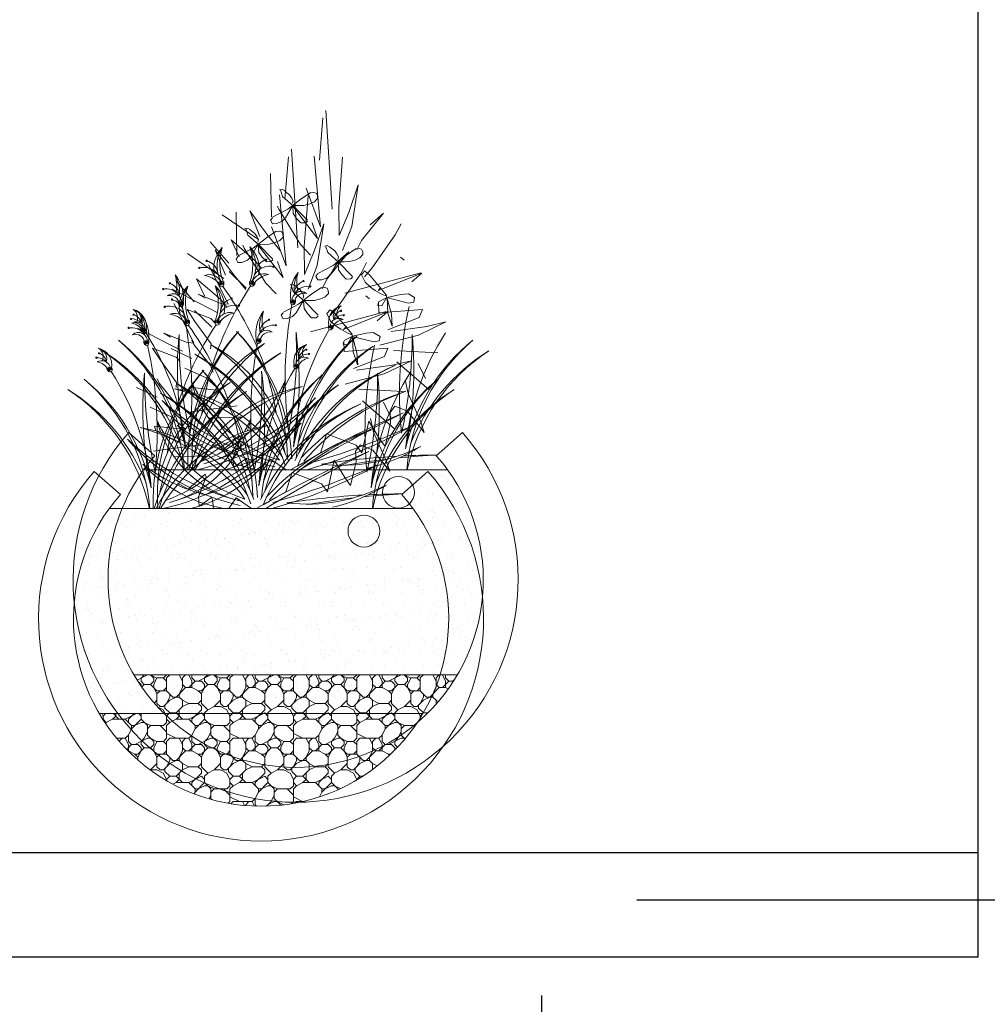
# Model space of a CAD drawing. Units: inches. Extents: x 89 to 490, y -59 to 378.
# Tile 15 of 20: x 429 to 460, y -28 to 3. Entities that reach past the tile are written whole.
import ezdxf

# ---------------------------------------------------------------- set-up
doc = ezdxf.new("R2010")
doc.units = ezdxf.units.IN
doc.header["$MEASUREMENT"] = 0
for name, color, linetype, lineweight in [('A-ANNO-DIMS', 2, 'Continuous', 18), ('L-PLNT', 94, 'Continuous', 18), ('L-PLNT-EDGE', 31, 'Continuous', 25)]:
    doc.layers.add(name, color=color, linetype=linetype, lineweight=lineweight)
doc.layers.add('fl', color=73, linetype='Continuous', lineweight=9, true_color=0xa3d166)
doc.styles.get("Standard").update_dxf_attribs({"font": 'arial.ttf'})
doc.dimstyles.get("Standard").update_dxf_attribs({"dimtxt": 6, "dimasz": 4, "dimexe": 3, "dimexo": 3, "dimgap": 0.09, "dimtad": 0, "dimtih": 1, "dimtoh": 1, "dimdec": 1, "dimzin": 0, "dimdsep": 46, "dimlunit": 3, "dimtxsty": 'Standard', "dimcen": 0.09, "dimadec": 0, "dimazin": 0, "dimtfac": 1, "dimtdec": 1, "dimtofl": 0, "dimtmove": 0, "dimatfit": 3, "dimfxl": 1, "dimtolj": 1, "dimtzin": 0, "dimarcsym": 0})

# ---------------------------------------------------------------- blocks, each defined once
blk = doc.blocks.new('1')
at = {"layer": 'fl'}
h = blk.add_hatch(dxfattribs=at)
h.set_pattern_fill('AR-SAND', color=256, scale=570.105873, style=0)
h.set_pattern_definition([(37.5, (-3711399.5, -832187.1), (-35.91288, 1098.49355), [0, -866.56093, 0, -969.17998, 0, -926.42204]), (7.5, (-3711399.5, -832187.1), (1008.9601, 1608.92205), [0, -467.48682, 0, -781.04505, 0, -299.30558]), (327.5, (-3712100.7, -832187.1), (1775.39056, 3.22626), [0, -285.05294, 0, -1026.19057, 0, -1339.7488]), (317.5, (-3712100.7, -832187.1), (1713.81043, 500.368), [0, -142.52647, 0, -672.72493, 0, -769.64293])])
h.paths.add_polyline_path([(227046, 19995, 0.298047), (226601, 10772), (241144, 10772, 0.298047), (240699, 19995)])
h.paths.add_polyline_path([(237778, 18976, -1), (239209, 18976, -1)], flags=16)
h = blk.add_hatch(dxfattribs=at)
h.set_pattern_fill('GHIAIA2', color=256, scale=2850.529365, style=0, pattern_type=2)
h.set_pattern_definition([(0, (-3711257, -832187), (2850.5294, 2850.5294), [855.1588, -997.6853, 142.5265, -855.1588]), (0, (-3710116.7, -831617), (2850.5294, 2850.5294), [142.5265, -712.6323, 570.1059, -1425.2647]), (0, (-3709689.2, -831474.5), (2850.5294, 2850.5294), [142.5265, -2708.0029]), (0, (-3710972, -831332), (2850.5294, 2850.5294), [570.1059, -2280.4235]), (0, (-3711257, -831047), (2850.5294, 2850.5294), [285.053, -2565.4764]), (0, (-3709261.6, -830761.8), (2850.5294, 2850.5294), [285.0529, -142.5265, 142.5265, -2280.4235]), (0, (-3710401.8, -830619.3), (2850.5294, 2850.5294), [427.5794, -2422.95]), (0, (-3711114.4, -830334.2), (2850.5294, 2850.5294), [285.053, -2565.4764]), (0, (-3709974.2, -830049.2), (2850.5294, 2850.5294), [142.5265, -855.1588, 427.5794, -1425.2647]), (0, (-3710544.3, -829906.7), (2850.5294, 2850.5294), [285.053, -2565.4764]), (0, (-3709546.6, -829764), (2850.5294, 2850.5294), [285.053, -2565.4764]), (0, (-3710116.7, -829621.6), (2850.5294, 2850.5294), [285.053, -2565.4764]), (0, (-3708976.5, -829479), (2850.5294, 2850.5294), [285.053, -2565.4764]), (90, (-3711399.5, -832187), (-2850.5294, 2850.5294), [570.1059, -142.5265, 285.05294, -1140.21175, 570.1059, -142.5265]), (90, (-3711257, -830334.2), (-2850.5294, 2850.5294), [142.5265, -2708.0029]), (90, (-3710829.4, -831189.4), (-2850.5294, 2850.5294), [285.0529, -570.1059, 142.5265, -1852.8441]), (90, (-3710686.9, -830761.8), (-2850.5294, 2850.5294), [285.0529, -570.1059, 427.5794, -1567.7912]), (90, (-3710259.3, -831474.5), (-2850.5294, 2850.5294), [142.5265, -1425.2647, 285.05294, -142.5265, 285.05294, -570.1059]), (90, (-3710116.7, -831759.5), (-2850.5294, 2850.5294), [142.5265, -2708.0029]), (90, (-3709831.7, -830904.3), (-2850.5294, 2850.5294), [142.5265, -142.5265, 427.5794, -2137.897]), (90, (-3709689.2, -831332), (-2850.5294, 2850.5294), [285.05294, -1140.21175, 142.5265, -142.5265, 142.5265, -997.6853]), (90, (-3709404, -832044.6), (-2850.5294, 2850.5294), [427.5794, -2422.95]), (90, (-3709119, -829906.7), (-2850.5294, 2850.5294), [142.5265, -142.5265, 142.5265, -2422.95]), (90, (-3708976.5, -830619.3), (-2850.5294, 2850.5294), [427.5794, -2422.95]), (90, (-3708620.2, -830833), (-2850.5294, 2850.5294), [142.5265, -2708.0029]), (45, (-3710401.8, -832187), (3e-13, 2850.5294), [201.561, -3829.6964]), (45, (-3710686.9, -829479), (3e-13, 2850.5294), [201.5609, -604.6828, 604.6828, -2620.3308]), (45, (-3710401.8, -829906.7), (3e-13, 2850.5294), [403.1219, -1007.8143, 201.5609, -2418.7601]), (45, (-3709831.7, -830049.2), (3e-13, 2850.5294), [403.1219, -1410.9408, 201.5609, -2015.6337]), (45, (-3710972, -831332), (3e-13, 2850.5294), [201.561, -3829.6964]), (45, (-3710259.3, -831332), (3e-13, 2850.5294), [604.6885, -3426.5688]), (45, (-3709689.2, -831046.9), (3e-13, 2850.5294), [201.5609, -1209.377, 201.5609, -2418.7584]), (45, (-3709261.6, -830761.8), (3e-13, 2850.5294), [403.1219, -3628.1354]), (45, (-3708691.5, -830761.8), (3e-13, 2850.5294), [403.1219, -3628.1354]), (45, (-3708691.5, -831617), (3e-13, 2850.5294), [201.561, -3829.6964]), (45, (-3708976.5, -830191.7), (3e-13, 2850.5294), [201.561, -3829.6964]), (45, (-3709261.6, -829764.1), (3e-13, 2850.5294), [201.561, -3829.6964]), (45, (-3708691.5, -829479), (3e-13, 2850.5294), [201.561, -3829.6964]), (45, (-3711399.5, -829479), (3e-13, 2850.5294), [201.561, -3829.6964]), (45, (-3709974.2, -830619.3), (3e-13, 2850.5294), [201.561, -3829.6964]), (45, (-3709689.2, -829479), (3e-13, 2850.5294), [201.5609, -1410.9408, 201.5609, -2217.1947]), (45, (-3710972, -831046.9), (3e-13, 2850.5294), [403.1219, -3628.1354]), (45, (-3710972, -830334.2), (3e-13, 2850.5294), [604.6828, -3426.5745]), (135, (-3711257, -831046.9), (-2850.5294, 3e-13), [302.3556, -3728.9016]), (135, (-3709689.2, -831189.4), (-2850.5294, 3e-13), [201.561, -3829.6964]), (135, (-3708834, -830761.8), (-2850.5294, 3e-13), [201.561, -3829.6964]), (135, (-3709831.7, -830191.7), (-2850.5294, 3e-13), [201.561, -3829.6964]), (135, (-3709689.2, -829764.1), (-2850.5294, 3e-13), [201.561, -3829.6964]), (135, (-3710116.7, -829621.6), (-2850.5294, 3e-13), [201.561, -3829.6964]), (135, (-3709546.6, -829764.1), (-2850.5294, 3e-13), [201.561, -3829.6964]), (135, (-3711257, -831474.5), (-2850.5294, 3e-13), [201.561, -3829.6964]), (135, (-3710686.9, -830476.8), (-2850.5294, 3e-13), [201.561, -3829.6964]), (135, (-3710686.9, -831332), (-2850.5294, 3e-13), [403.1219, -3628.1354]), (135, (-3710116.7, -831617), (-2850.5294, 3e-13), [403.1219, -3628.1354]), (135, (-3708976.5, -830049.2), (-2850.5294, 3e-13), [403.1219, -3628.1354]), (135, (-3709831.7, -830761.8), (-2850.5294, 3e-13), [201.561, -3829.6964]), (135, (-3709404.1, -831617), (-2850.5294, 3e-13), [403.1219, -2418.754, 201.5609, -1007.8205]), (135, (-3711114.4, -830334.2), (-2850.5279, 0.0014), [403.1219, -806.2514, 403.1219, -2418.7621]), (135, (-3711399.5, -831902), (-2850.5294, 3e-13), [403.06485, -1007.9472, 403.06485, -1007.9472, 201.5324, -1007.7008]), (26.56505, (-3710401.8, -831331.9), (2850.52937, 1e-07), [637.3784, -318.6892, 318.6892, -5099.2207]), (26.56505, (-3709974.2, -829621.6), (2850.52937, 1e-07), [637.3784, -5736.599]), (26.56505, (-3709974.2, -831617), (2850.52937, 1e-07), [318.6892, -6055.2882]), (26.56505, (-3711257, -831474.5), (2850.52937, 1e-07), [318.6892, -6055.2882]), (26.56505, (-3710686.9, -830761.8), (2850.52937, 1e-07), [318.6892, -6055.2882]), (26.56505, (-3711257, -830476.8), (2850.52937, 1e-07), [318.6892, -6055.2882]), (63.43495, (-3710829.4, -830191.7), (1e-07, 2850.52937), [318.6892, -6055.2882]), (63.43495, (-3709831.7, -830191.7), (1e-07, 2850.52937), [318.6892, -6055.2882]), (63.43495, (-3709546.6, -832187.1), (1e-07, 2850.52937), [318.6892, -6055.2882]), (63.43495, (-3711399.5, -830619.3), (1e-07, 2850.52937), [318.6892, -6055.2882]), (63.43495, (-3710259.3, -832044.6), (1e-07, 2850.52937), [318.6892, -2230.8243, 318.6892, -3505.7748]), (116.56505, (-3710686.9, -829621.6), (-1e-07, 2850.52937), [318.6892, -6055.2882]), (116.56505, (-3708976.5, -830191.7), (-1e-07, 2850.52937), [318.6892, -6055.2882]), (116.56505, (-3710259.3, -829621.6), (-1e-07, 2850.52937), [318.6892, -6055.2882]), (116.56505, (-3711399.5, -831189.4), (-1e-07, 2850.52937), [318.6892, -6055.2882]), (153.43495, (-3709261.6, -831617), (-2850.52937, 1e-07), [318.6892, -6055.2882]), (153.43495, (-3708691.5, -830904.3), (-2850.52937, 1e-07), [318.6892, -6055.2882]), (153.43495, (-3710401.8, -830619.3), (-2850.52937, 1e-07), [318.6892, -6055.2882]), (153.43495, (-3709974.2, -830049.2), (-2850.52937, 1e-07), [318.6892, -6055.2882]), (153.43495, (-3708976.5, -829479.1), (-2850.52937, 1e-07), [318.6892, -6055.2882]), (153.43495, (-3710971.9, -832187.1), (-2850.52937, 1e-07), [478.0338, -5895.9437])])
h.paths.add_polyline_path([(241144, 10772), (226601, 10772, 0.572327)])
for p, q in [((235236, 36144), (235518, 31709)), ((234942, 33904), (235098, 35808)), ((234701, 34090), (234994, 30911)), ((235981, 34049), (235808, 31793)), ((232784, 31366), (232750, 33316)), ((236260, 31559), (236691, 32796)), ((236691, 32796), (236393, 30924)), ((233148, 32578), (233261, 32601)), ((233186, 32582), (233280, 32279)), ((233261, 32601), (233366, 32540)), ((233366, 32540), (233472, 32449)), ((233472, 32449), (233598, 32357)), ((233598, 32357), (233684, 32223)), ((234117, 32169), (234551, 32462)), ((234994, 30911), (234346, 32658)), ((234688, 32459), (234584, 32447)), ((234803, 32430), (234688, 32459)), ((234857, 32317), (234803, 32430)), ((234859, 32192), (234857, 32317)), ((233280, 32279), (233766, 31852)), ((233521, 31704), (234117, 32169)), ((233684, 32223), (233759, 32089)), ((233759, 32089), (233730, 31974)), ((234023, 31865), (234241, 31879)), ((234241, 31879), (234510, 31946)), ((234510, 31946), (234716, 32044)), ((234716, 32044), (234859, 32192)), ((232201, 30339), (230567, 31451)), ((232269, 30478), (231813, 31629)), ((231813, 31629), (232629, 30518)), ((232839, 31348), (233521, 31704)), ((233056, 31838), (233117, 31701)), ((233117, 31701), (234087, 30123)), ((233419, 31324), (233732, 31860)), ((233743, 31839), (234860, 30385)), ((233743, 31839), (233769, 31507)), ((233763, 31871), (234023, 31865)), ((233766, 31852), (234400, 31206)), ((233769, 31507), (233918, 31291)), ((235808, 31793), (235824, 30516)), ((235824, 30516), (236260, 31559)), ((237817, 31528), (236831, 30300)), ((237224, 31008), (237817, 31528)), ((232826, 31324), (232745, 31208)), ((232745, 31208), (232831, 31053)), ((232831, 31053), (233008, 31057)), ((233008, 31057), (233256, 31155)), ((233256, 31155), (233419, 31324)), ((233918, 31291), (234109, 31086)), ((234109, 31086), (234317, 31100)), ((234317, 31100), (234399, 31174)), ((234860, 30385), (234611, 31094)), ((238611, 31055), (238351, 30546)), ((236393, 30924), (235985, 29855)), ((238351, 30546), (237318, 29067)), ((230034, 30240), (230871, 29280)), ((231328, 29557), (230969, 30323)), ((230969, 30323), (232057, 29387)), ((232629, 30518), (233180, 29842)), ((234087, 30123), (234548, 29639)), ((236831, 30300), (236623, 29876)), ((235183, 30051), (235297, 30073)), ((235221, 30054), (235315, 29752)), ((235297, 30073), (235402, 30013)), ((235315, 29752), (235802, 29324)), ((235402, 30013), (235508, 29921)), ((235508, 29921), (235634, 29830)), ((235634, 29830), (235719, 29696)), ((235719, 29696), (235795, 29562)), ((236152, 29642), (236587, 29934)), ((236724, 29932), (236620, 29920)), ((236839, 29903), (236724, 29932)), ((236752, 29516), (236895, 29664)), ((236893, 29789), (236839, 29903)), ((236895, 29664), (236893, 29789)), ((232057, 29387), (232318, 29063)), ((235454, 28796), (235767, 29332)), ((235557, 29177), (236152, 29642)), ((235795, 29562), (235765, 29447)), ((235778, 29312), (235805, 28979)), ((235798, 29343), (236058, 29338)), ((235802, 29324), (236435, 28679)), ((236058, 29338), (236276, 29352)), ((236276, 29352), (236546, 29419)), ((236546, 29419), (236752, 29516)), ((238579, 29554), (238750, 29421)), ((230367, 28413), (229952, 29204)), ((230879, 28903), (231654, 28151)), ((234862, 28796), (234781, 28681)), ((234875, 28820), (235557, 29177)), ((235291, 28627), (235454, 28796)), ((235805, 28979), (235954, 28763)), ((239495, 28850), (236091, 27935)), ((236834, 28758), (236972, 28931)), ((237318, 29067), (236970, 28666)), ((236972, 28931), (237195, 28756)), ((237575, 28048), (239548, 28837)), ((239548, 28837), (239089, 28433)), ((230845, 27429), (230367, 28413)), ((234781, 28681), (234867, 28526)), ((234867, 28526), (235043, 28529)), ((235043, 28529), (235291, 28627)), ((235954, 28763), (236145, 28559)), ((236145, 28559), (236352, 28573)), ((236352, 28573), (236434, 28647)), ((236997, 28419), (236834, 28758)), ((237240, 28194), (236997, 28419)), ((237948, 27851), (237192, 28756)), ((230346, 27064), (228328, 28107)), ((237454, 28055), (237240, 28194)), ((237766, 27876), (237454, 28055)), ((237709, 28191), (237575, 28048)), ((238940, 27902), (238593, 27872)), ((238941, 27896), (239218, 27731)), ((229808, 27699), (229497, 27883)), ((229497, 27883), (230511, 27473)), ((230511, 27473), (230845, 27429)), ((237593, 27520), (237565, 27376)), ((237593, 27520), (237609, 27049)), ((237991, 27741), (237603, 27547)), ((237750, 27365), (237975, 27748)), ((237951, 27807), (237766, 27876)), ((238179, 26992), (237948, 27851)), ((238014, 27032), (237983, 27728)), ((238593, 27872), (237991, 27741)), ((238935, 27487), (238028, 27717)), ((239181, 27525), (238935, 27487)), ((239218, 27731), (239181, 27525)), ((229344, 26656), (228992, 27199)), ((228992, 27199), (230062, 26791)), ((237565, 27376), (237750, 27365)), ((237609, 27049), (239576, 27199)), ((238207, 26450), (238014, 27032)), ((239576, 27199), (239422, 26833)), ((230073, 25653), (229344, 26656)), ((230062, 26791), (230235, 26603)), ((239422, 26833), (238024, 26285)), ((238219, 26460), (238179, 26992)), ((240626, 26636), (239401, 26044)), ((239775, 26431), (240626, 26636)), ((238163, 26213), (239775, 26431)), ((229296, 25626), (229206, 25818)), ((239401, 26044), (237652, 25586)), ((228272, 25437), (229202, 24992)), ((230050, 24680), (229296, 25626)), ((230052, 25430), (230073, 25653)), ((238273, 25359), (240270, 25251)), ((238425, 24839), (239872, 23581)), ((229847, 24117), (228888, 24557)), ((230172, 24378), (230050, 24680)), ((239381, 24776), (239710, 24093)), ((230478, 23555), (229847, 24117)), ((238795, 24034), (238927, 23427)), ((229147, 23482), (229084, 23702)), ((229084, 23702), (230059, 23597)), ((230107, 23015), (229147, 23482)), ((230059, 23597), (230478, 23555)), ((238927, 23427), (239498, 22141)), ((229039, 22577), (231240, 22872)), ((230219, 22991), (230107, 23015)), ((238335, 22851), (238123, 22566)), ((238899, 22620), (238335, 22851)), ((239653, 21674), (238899, 22620)), ((230908, 22348), (229936, 22315)), ((231463, 22367), (230908, 22348)), ((231216, 22275), (231463, 22367)), ((237164, 22172), (236851, 20745)), ((237635, 21383), (237164, 22172)), ((238123, 22566), (238139, 22094)), ((239498, 22141), (239653, 21674)), ((238139, 22094), (237897, 21031)), ((227550, 20624), (226375, 21661)), ((231352, 21530), (230597, 20865)), ((231053, 20519), (231411, 21421)), ((231411, 21421), (231352, 21530)), ((235266, 21608), (234991, 20737)), ((236589, 21097), (235266, 21608)), ((237897, 21031), (237635, 21383)), ((240196, 20624), (241371, 21661)), ((230597, 20865), (230116, 21126)), ((236851, 20745), (236589, 21097)), ((231095, 20104), (231053, 20519)), ((231638, 20484), (231095, 20104)), ((231696, 20402), (231638, 20484)), ((231736, 19995), (231696, 20402)), ((232750, 20466), (232416, 19995)), ((233443, 19995), (232750, 20466)), ((234991, 20737), (233649, 19995)), ((227046, 19995), (240699, 19995)), ((226601, 10772), (241144, 10772))]:
    blk.add_line(p, q, dxfattribs=at)
blk.add_circle((238494, 18976), 715, dxfattribs=at)
for centre, radius, start, end in [((231547, 29038), 1357, 135.5632, 193.7293), ((231825, 29181), 1486, 147.096, 209.2874), ((232883, 29270), 2415, 162.6858, 201.1197), ((230595, 29157), 1486, 332.7126, 34.904), ((230878, 29024), 1357, 348.2707, 46.4368), ((229534, 29208), 2415, 340.8803, 19.3142), ((229870, 29388), 30.3, 11.802, 191.802), ((229870, 29388), 30.3, 191.802, 11.802), ((229720, 28734), 665, 13.7128, 76.1437), ((232714, 28784), 665, 105.8563, 168.2872), ((232542, 29431), 30.3, 350.198, 170.198), ((232542, 29431), 30.3, 170.198, 350.198), ((229545, 29064), 30.3, 11.802, 191.802), ((229744, 28283), 809, 35.6636, 106.404), ((229545, 29064), 30.3, 191.802, 11.802), ((232463, 28230), 577, 70.2507, 170.8138), ((232707, 28332), 809, 75.596, 146.3364), ((232857, 27714), 1078, 100.6373, 137.9791), ((232878, 29119), 30.3, 170.198, 350.198), ((232878, 29119), 30.3, 350.198, 170.198), ((235268, 27859), 1631, 142.1725, 190.5866), ((235289, 28157), 1486, 151.8051, 190.4904), ((235410, 28441), 1490, 163.721, 197.6936), ((228220, 28372), 26.2, 7.5892, 187.5892), ((228220, 28372), 26.2, 187.5892, 7.5892), ((227972, 27703), 710, 16.8512, 68.8014), ((227201, 27715), 1631, 351.4134, 39.8275), ((227038, 28292), 1490, 344.3064, 18.279), ((227169, 28013), 1486, 351.5096, 30.1949), ((229991, 28190), 577, 11.1862, 111.7493), ((229615, 27661), 1078, 44.0209, 81.3627), ((230581, 28404), 191, 172.3781, 246.6066), ((230746, 28600), 394, 205.7422, 233.1344), ((230840, 28459), 373, 178.723, 207.7572), ((230930, 28612), 485, 197.3111, 219.7508), ((230165, 28193), 459, 16.3461, 37.9549), ((231390, 28535), 864, 184.0141, 195.6693), ((229958, 28569), 693, 339.0728, 350.8866), ((230259, 28375), 393, 348.1534, 12.4334), ((232189, 28406), 393, 169.5666, 193.8466), ((232482, 28610), 693, 191.1134, 202.9272), ((232288, 28227), 459, 144.0451, 165.6539), ((231053, 28526), 864, 346.3307, 357.9859), ((231510, 28619), 485, 322.2492, 344.6889), ((231604, 28469), 373, 334.2428, 3.277), ((231693, 28614), 394, 308.8656, 336.2578), ((231866, 28423), 191, 295.3934, 9.6219), ((234498, 27820), 710, 113.1986, 165.1488), ((234226, 28480), 26.2, 354.4108, 174.4108), ((234226, 28480), 26.2, 174.4108, 354.4108), ((227920, 28114), 26.2, 7.5892, 187.5892), ((228033, 27332), 792, 39.5069, 100.1323), ((227920, 28114), 26.2, 187.5892, 7.5892), ((228360, 27505), 401, 357.4175, 130.8703), ((243581, 20409), 14112, 146.2244, 163.2125), ((230547, 28319), 100, 245.3588, 345.3239), ((219152, 19986), 14112, 18.7875, 35.7756), ((231903, 28340), 100, 196.6761, 296.6412), ((234116, 27608), 401, 51.1297, 184.5825), ((234449, 27447), 792, 81.8677, 142.4931), ((234262, 27502), 431, 75.8945, 175.0168), ((234535, 28232), 26.2, 354.4108, 174.4108), ((234535, 28232), 26.2, 174.4108, 354.4108), ((228218, 27394), 431, 6.9832, 106.1055), ((228771, 27479), 165, 168.1654, 242.3938), ((228926, 27638), 341, 201.5294, 228.9216), ((228998, 27510), 323, 174.5103, 203.5444), ((229085, 27636), 419, 193.0983, 215.538), ((229477, 27541), 747, 179.8013, 191.4565), ((228399, 27323), 397, 12.1333, 33.7421), ((228245, 27661), 599, 334.86, 346.6738), ((228491, 27474), 340, 343.9406, 8.2206), ((233986, 27573), 340, 173.7794, 198.0594), ((234226, 27768), 599, 195.3262, 207.14), ((233744, 27498), 86.5, 200.8889, 300.854), ((234083, 27425), 397, 148.2579, 169.8667), ((232999, 27605), 747, 350.5435, 2.1987), ((233387, 27714), 419, 326.462, 348.9017), ((233478, 27591), 323, 338.4556, 7.4897), ((233546, 27721), 341, 313.0784, 340.4706), ((233706, 27568), 165, 299.6062, 13.8346), ((226443, 26721), 493, 342.816, 75.0201), ((226319, 26821), 453, 335.7976, 56.2278), ((226384, 26438), 782, 349.633, 76.1366), ((228736, 27408), 86.5, 241.146, 341.1111), ((211209, 23423), 17995, 354.2791, 12.5427), ((251399, 24127), 17995, 169.4573, 187.7209), ((236129, 26611), 782, 105.8634, 192.367), ((236059, 26892), 493, 106.9799, 199.184), ((236234, 26525), 710, 116.6992, 157.9158), ((236180, 26996), 453, 125.7722, 206.2024), ((235907, 27134), 26.2, 162.351, 342.351), ((235907, 27134), 26.2, 342.351, 162.351), ((256536, 23423), 17995, 167.4573, 185.7209), ((226473, 26770), 26.2, 19.649, 199.649), ((226473, 26770), 26.2, 199.649, 19.649), ((226419, 25998), 792, 50.416, 87.3549), ((226705, 26237), 398, 9.2042, 120.225), ((226411, 25929), 659, 27.9293, 81.8071), ((226587, 26968), 26.2, 19.649, 199.649), ((226587, 26968), 26.2, 199.649, 19.649), ((226281, 26348), 710, 24.0842, 65.3008), ((235814, 26399), 398, 61.775, 172.7958), ((236119, 26101), 659, 100.1929, 154.0707), ((236109, 26170), 792, 94.6451, 131.584), ((236028, 26940), 26.2, 162.351, 342.351), ((236028, 26940), 26.2, 342.351, 162.351), ((227110, 26296), 165, 180.2252, 254.4537), ((227228, 26483), 341, 213.5892, 240.9815), ((227326, 26374), 323, 186.5701, 215.6042), ((227384, 26515), 419, 205.1582, 227.5978), ((226779, 26066), 397, 24.1932, 45.802), ((227787, 26504), 747, 191.8611, 203.5164), ((227090, 26219), 86.5, 253.2058, 353.1709), ((217426, 19891), 11552, 5.151, 32.7872), ((226557, 26364), 599, 346.9198, 358.7337), ((226837, 26233), 340, 356.0005, 20.2804), ((237706, 20343), 8686, 137.4916, 182.296), ((237741, 20623), 8526, 139.0392, 184.2242), ((224981, 20403), 8526, 0.703, 42.9608), ((225026, 20124), 8686, 2.3901, 44.5084), ((214488, 25343), 19422, 349.2183, 2.4529), ((245310, 20381), 11552, 149.2128, 176.849), ((216951, 23979), 17083, 350.0105, 7.3826), ((235683, 26390), 340, 161.7196, 185.9995), ((235430, 26368), 86.5, 188.8291, 288.7942), ((235958, 26531), 599, 183.2663, 195.0802), ((235747, 26225), 397, 136.198, 157.8068), ((234724, 26628), 747, 338.4836, 350.1389), ((235126, 26653), 419, 314.4022, 336.8418), ((235408, 26443), 165, 287.5463, 1.7748), ((235190, 26514), 323, 326.3958, 355.4299), ((235283, 26627), 341, 301.0185, 328.4108), ((250320, 19891), 11552, 147.2128, 174.849), ((220372, 19333), 8526, 4.4514, 49.4547), ((220448, 19061), 8686, 12.4122, 51.0023), ((245642, 24477), 17083, 174.6174, 191.9895), ((248056, 25926), 19422, 179.5471, 192.7817), ((242318, 19446), 8686, 130.9977, 169.5878), ((242385, 19720), 8526, 132.5453, 174.8032), ((219689, 25926), 19422, 347.2183, 0.4529), ((222104, 24477), 17083, 348.0105, 5.3826), ((247297, 19061), 8686, 128.9977, 167.5878), ((247373, 19333), 8526, 130.5453, 175.5486), ((220516, 18210), 8526, 12.0849, 56.7339), ((220626, 17950), 8686, 21.5651, 58.2814), ((238130, 17111), 9510, 121.1471, 162.3489), ((235946, 19736), 6867, 120.3536, 167.8423), ((238207, 17430), 9279, 122.567, 163.9531), ((237105, 19238), 7918, 125.7805, 169.1581), ((225665, 19041), 7918, 12.8419, 56.2195), ((226807, 19579), 6867, 14.1577, 61.6464), ((242180, 18329), 8686, 123.7186, 160.4349), ((242280, 18592), 8526, 125.2661, 165.1679), ((247230, 18210), 8526, 123.2661, 167.9151), ((247120, 17950), 8686, 121.7186, 158.4349), ((224715, 16880), 9510, 21.708, 60.8529), ((224627, 17196), 9279, 18.8656, 59.433), ((241697, 16676), 8686, 112.5744, 154.7193), ((241847, 16915), 8526, 114.122, 157.6363), ((234084, 25273), 5074, 194.9574, 201.3849), ((235856, 27195), 7415, 205.8333, 210.9541), ((242175, 20950), 12610, 165.3183, 172.932), ((220539, 20575), 12610, 9.068, 16.6817), ((226636, 27031), 7415, 331.0459, 336.1667), ((228474, 25172), 5074, 340.6151, 347.0426), ((227307, 16498), 7223, 34.1912, 81.04), ((226269, 15391), 8521, 36.1662, 75.2917), ((235553, 16639), 7223, 100.96, 152.3132), ((236629, 15569), 8521, 106.7083, 148.7079), ((242176, 13079), 10968, 107.7857, 137.2506), ((242527, 13226), 10941, 109.7712, 139.1936), ((235849, 31659), 11695, 226.9943, 255.7863), ((234889, 29252), 9328, 221.2139, 257.9277), ((234084, 25273), 5074, 202.7107, 257.3947), ((227531, 29121), 9328, 281.9445, 320.7861), ((227499, 26311), 6310, 289.2472, 331.4766), ((235019, 26446), 6310, 210.5234, 252.7528), ((228474, 25172), 5074, 284.6053, 339.2893), ((226488, 31492), 11695, 286.2137, 315.0057), ((257604, -20830), 47319, 113.5344, 119.9765), ((266096, -32559), 61541, 116.42332, 121.34648), ((233192, 27894), 7507, 231.8384, 256.0141), ((233324, 26366), 6472, 222.5197, 259.8837), ((229196, 26291), 6472, 283.378, 319.4803), ((229274, 27823), 7507, 285.9859, 310.1616), ((225434, 52492), 33452, 285.56, 294.0219), ((228714, 40229), 21012, 285.7446, 299.4741), ((233873, 15043), 10001, 138.5688, 41.4312), ((235941, 28021), 7831, 263.3334, 297.0085), ((235282, 27872), 8025, 282.9751, 301.6856), ((233873, 15043), 8433, 138.5688, 41.4312), ((240331, -13838), 34490, 93.1391, 98.8421), ((241951, -13820), 34514, 96.5562, 99.7904), ((241951, -13820), 34514, 92.8276, 95.7392), ((240331, -13838), 34490, 90.1381, 92.7056)]:
    blk.add_arc(centre, radius, start, end, dxfattribs=at)
blk = doc.blocks.new('Plantation')
at = {"layer": 'fl', "xscale": 0.0006983696904879, "yscale": 0.0006983696904879, "zscale": 0.0006983696904879}
for p in [(498.581, 9.546), (497.497, 8.328)]:
    blk.add_blockref('1', p, dxfattribs=at)
blk = doc.blocks.new('*D46')
at = {"layer": 'A-ANNO-DIMS', "color": 0, "lineweight": -2, "transparency": 16777216}
for p, q in [((277.443, -27.866), (277.443, -53.11)), ((445.739, -27.866), (445.739, -53.11)), ((281.443, -50.11), (332.892, -50.11)), ((441.739, -50.11), (390.289, -50.11))]:
    blk.add_line(p, q, dxfattribs=at)
at = {"layer": 'A-ANNO-DIMS', "color": 0, "transparency": 16777216}
for points in [[(281.443, -49.443), (281.443, -50.777), (277.443, -50.11)], [(441.739, -49.443), (441.739, -50.777), (445.739, -50.11)]]:
    blk.add_solid(points, dxfattribs=at)
at = {"layer": 'Defpoints', "color": 0, "transparency": 16777216}
for p in [(277.443, -24.866), (445.739, -24.866), (445.739, -50.11)]:
    blk.add_point(p, dxfattribs=at)
at = {"layer": 'A-ANNO-DIMS', "color": 0, "transparency": 16777216, "insert": (361.591, -50.11), "char_height": 6, "attachment_point": 5}
blk.add_mtext('\\A1;PLANTING 168', dxfattribs=at)
blk = doc.blocks.new('*D47')
at = {"layer": 'A-ANNO-DIMS', "color": 0, "lineweight": -2, "transparency": 16777216}
for p, q in [((448.739, 7.78), (473.983, 7.78)), ((470.983, 3.78), (470.983, -5.387)), ((470.983, -20.866), (470.983, -11.698)), ((448.739, -24.866), (473.983, -24.866))]:
    blk.add_line(p, q, dxfattribs=at)
at = {"layer": 'A-ANNO-DIMS', "color": 0, "transparency": 16777216}
for points in [[(470.316, 3.78), (471.65, 3.78), (470.983, 7.78)], [(470.316, -20.866), (471.65, -20.866), (470.983, -24.866)]]:
    blk.add_solid(points, dxfattribs=at)
at = {"layer": 'Defpoints', "color": 0, "transparency": 16777216}
for p in [(445.739, 7.78), (470.983, 7.78), (445.739, -24.866)]:
    blk.add_point(p, dxfattribs=at)
at = {"layer": 'A-ANNO-DIMS', "color": 0, "transparency": 16777216, "insert": (470.983, -8.543), "char_height": 6, "attachment_point": 5}
blk.add_mtext('\\A1;33', dxfattribs=at)
blk = doc.blocks.new('*D48')
at = {"layer": 'A-ANNO-DIMS', "color": 0, "lineweight": -2, "transparency": 16777216}
for p, q in [((127.441, 10.741), (127.441, -49.809)), ((459.441, -29.659), (459.441, -49.809)), ((131.441, -46.809), (286.756, -46.809)), ((455.441, -46.809), (300.127, -46.809))]:
    blk.add_line(p, q, dxfattribs=at)
at = {"layer": 'A-ANNO-DIMS', "color": 0, "transparency": 16777216}
for points in [[(131.441, -46.143), (131.441, -47.476), (127.441, -46.809)], [(455.441, -46.143), (455.441, -47.476), (459.441, -46.809)]]:
    blk.add_solid(points, dxfattribs=at)
at = {"layer": 'Defpoints', "color": 0, "transparency": 16777216}
for p in [(127.441, 13.741), (459.441, -26.659), (459.441, -46.809)]:
    blk.add_point(p, dxfattribs=at)
at = {"layer": 'A-ANNO-DIMS', "color": 0, "transparency": 16777216, "insert": (293.441, -46.809), "char_height": 6, "attachment_point": 5}
blk.add_mtext('\\A1;332', dxfattribs=at)
blk = doc.blocks.new('*D49')
at = {"layer": 'A-ANNO-DIMS', "color": 0, "lineweight": -2, "transparency": 16777216}
for p, q in [((462.441, 353.741), (482.591, 353.741)), ((479.591, 349.741), (479.591, 166.696)), ((479.591, -22.659), (479.591, 160.385)), ((462.441, -26.659), (482.591, -26.659))]:
    blk.add_line(p, q, dxfattribs=at)
at = {"layer": 'A-ANNO-DIMS', "color": 0, "transparency": 16777216}
for points in [[(478.925, 349.741), (480.258, 349.741), (479.591, 353.741)], [(478.925, -22.659), (480.258, -22.659), (479.591, -26.659)]]:
    blk.add_solid(points, dxfattribs=at)
at = {"layer": 'Defpoints', "color": 0, "transparency": 16777216}
for p in [(459.441, 353.741), (479.591, 353.741), (459.441, -26.659)]:
    blk.add_point(p, dxfattribs=at)
at = {"layer": 'A-ANNO-DIMS', "color": 0, "transparency": 16777216, "insert": (479.591, 163.541), "char_height": 6, "attachment_point": 5}
blk.add_mtext('\\A1;380.4', dxfattribs=at)

msp = doc.modelspace()

# ---------------------------------------------------------------- linework, layer by layer
at = {"layer": 'L-PLNT-EDGE'}
for p, q in [((459.4414, 12.3406), (459.4414, -26.6594)), ((459.4414, -23.3886), (265.4414, -23.3886)), ((459.4414, -26.6594), (265.4414, -26.6594))]:
    msp.add_line(p, q, dxfattribs=at)

# ---------------------------------------------------------------- block references
at = {"layer": 'L-PLNT'}
msp.add_blockref('Plantation', (-223.8856, -34.8668), dxfattribs=at)

# ---------------------------------------------------------------- dimensions: what is measured, and where the dimension line sits
at = {"layer": 'A-ANNO-DIMS'}
for base, p1, p2, override, picture, middle in [((479.5914, 353.7413), (459.4414, -26.6594), (459.4414, 353.7413), {"dimdec": 1, "dimlfac": 1, "dimrnd": 0, "dimzin": 0, "dimdsep": 46, "dimlunit": 2}, '*D49', (479.5914, 163.5409)), ((470.9829, 7.78), (445.7386, -24.8656), (445.7386, 7.78), {"dimdec": 0, "dimlfac": 1, "dimrnd": 0, "dimzin": 0, "dimdsep": 46, "dimlunit": 2}, '*D47', (470.9829, -8.5428))]:
    dim = msp.add_linear_dim(base=base, p1=p1, p2=p2, angle=90, dimstyle='Standard', override=override, dxfattribs=at)
    dim.commit()
    dim.dimension.update_dxf_attribs({"geometry": picture, "text_midpoint": middle})
dim = msp.add_linear_dim(base=(459.4414, -46.8094), p1=(127.4414, 13.7413), p2=(459.4414, -26.6594), dimstyle='Standard', override={"dimdec": 0, "dimlfac": 1, "dimrnd": 0, "dimzin": 0, "dimdsep": 46, "dimlunit": 2}, dxfattribs=at)
dim.commit()
dim.dimension.update_dxf_attribs({"geometry": '*D48', "text_midpoint": (293.4414, -46.8094)})
dim = msp.add_linear_dim(base=(445.7386, -50.11), p1=(277.443, -24.8656), p2=(445.7386, -24.8656), text='PLANTING <>', dimstyle='Standard', override={"dimdec": 0, "dimlfac": 1, "dimrnd": 0, "dimzin": 0, "dimdsep": 46, "dimlunit": 2}, dxfattribs=at)
dim.commit()
dim.dimension.update_dxf_attribs({"geometry": '*D46', "text_midpoint": (361.5908, -50.11)})

doc.saveas('drawing.dxf')
